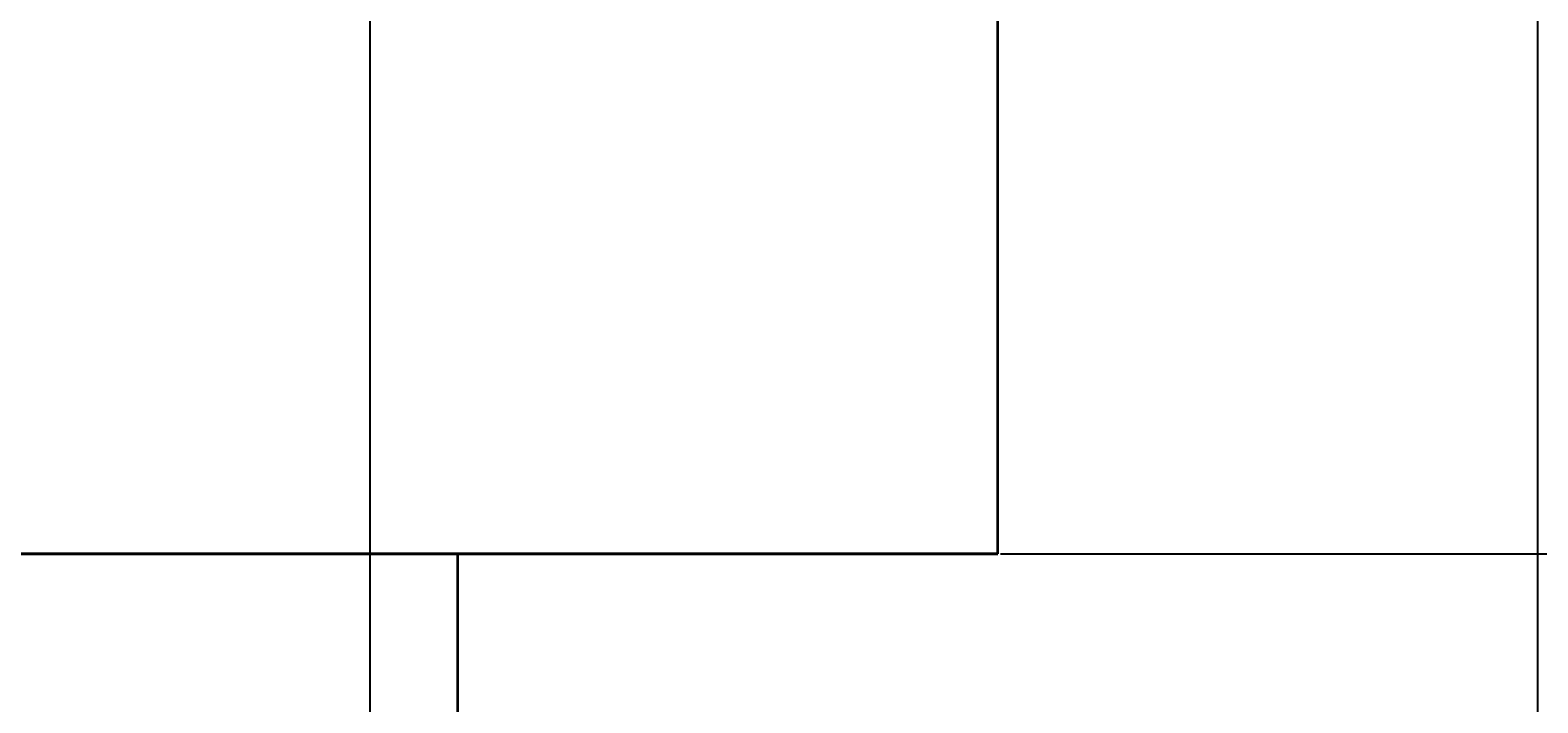
# Model space of a CAD drawing. Units: inches. Extents: x -6 to 289, y -8 to 323.
# Tile 64 of 107: x 238 to 271, y 124 to 139. Entities that reach past the tile are written whole.
import ezdxf

# ---------------------------------------------------------------- set-up
doc = ezdxf.new("R2010")
doc.units = ezdxf.units.IN
doc.header["$MEASUREMENT"] = 0
doc.layers.add('A-ANNO-DIMS', color=2, linetype='Continuous', lineweight=18)
doc.layers.add('A-ELEV', color=7, linetype='Continuous', lineweight=35)
doc.styles.get("Standard").update_dxf_attribs({"font": 'arial.ttf'})
doc.dimstyles.get("Standard").update_dxf_attribs({"dimtxt": 0.18, "dimasz": 0.18, "dimexe": 0.18, "dimexo": 0.0625, "dimgap": 0.09, "dimtad": 0, "dimtih": 1, "dimtoh": 1, "dimdec": 4, "dimzin": 0, "dimdsep": 46, "dimtxsty": 'Standard', "dimcen": 0.09, "dimadec": 0, "dimazin": 0, "dimtfac": 1, "dimtdec": 4, "dimtofl": 0, "dimtmove": 0, "dimatfit": 3, "dimfxl": 1, "dimtolj": 1, "dimtzin": 0, "dimarcsym": 0})

# ---------------------------------------------------------------- blocks, each defined once
blk = doc.blocks.new('*D15')
at = {"layer": 'A-ANNO-DIMS', "color": 0, "lineweight": -2, "transparency": 16777216}
for p, q in [((247.164, 162.411), (247.164, 322.969)), ((247.344, 322.789), (258.944, 322.789)), ((270.984, 322.789), (259.384, 322.789)), ((271.164, 7.351), (271.164, 322.969))]:
    blk.add_line(p, q, dxfattribs=at)
at = {"layer": 'A-ANNO-DIMS', "color": 0, "transparency": 16777216}
for points in [[(247.344, 322.819), (247.344, 322.759), (247.164, 322.789)], [(270.984, 322.819), (270.984, 322.759), (271.164, 322.789)]]:
    blk.add_solid(points, dxfattribs=at)
at = {"layer": 'Defpoints', "color": 0, "transparency": 16777216}
for p in [(271.164, 322.789), (247.164, 162.348), (271.164, 7.289)]:
    blk.add_point(p, dxfattribs=at)
at = {"layer": 'A-ANNO-DIMS', "color": 0, "transparency": 16777216, "insert": (259.164, 322.789), "char_height": 0.18, "attachment_point": 5}
blk.add_mtext('\\A1;24', dxfattribs=at)
blk = doc.blocks.new('*D23')
at = {"layer": 'A-ANNO-DIMS', "color": 0, "lineweight": -2, "transparency": 16777216}
for p, q in [((259.226, 127.289), (288.653, 127.289)), ((288.473, 127.109), (288.473, 67.471)), ((288.473, 7.469), (288.473, 67.107)), ((271.226, 7.289), (288.653, 7.289))]:
    blk.add_line(p, q, dxfattribs=at)
at = {"layer": 'A-ANNO-DIMS', "color": 0, "transparency": 16777216}
for points in [[(288.443, 127.109), (288.503, 127.109), (288.473, 127.289)], [(288.443, 7.469), (288.503, 7.469), (288.473, 7.289)]]:
    blk.add_solid(points, dxfattribs=at)
at = {"layer": 'Defpoints', "color": 0, "transparency": 16777216}
for p in [(259.164, 127.289), (288.473, 127.289), (271.164, 7.289)]:
    blk.add_point(p, dxfattribs=at)
at = {"layer": 'A-ANNO-DIMS', "color": 0, "transparency": 16777216, "insert": (288.473, 67.289), "char_height": 0.18, "attachment_point": 5}
blk.add_mtext('\\A1;120', dxfattribs=at)
blk = doc.blocks.new('*D81')
at = {"layer": 'A-ANNO-DIMS', "color": 0, "lineweight": -2, "transparency": 16777216}
for p, q in [((230.292, 68.842), (230.292, 322.969)), ((230.472, 322.789), (237.298, 322.789)), ((245.035, 322.789), (238.208, 322.789)), ((245.215, 66.286), (245.215, 322.969))]:
    blk.add_line(p, q, dxfattribs=at)
at = {"layer": 'A-ANNO-DIMS', "color": 0, "transparency": 16777216}
for points in [[(230.472, 322.819), (230.472, 322.759), (230.292, 322.789)], [(245.035, 322.819), (245.035, 322.759), (245.215, 322.789)]]:
    blk.add_solid(points, dxfattribs=at)
at = {"layer": 'Defpoints', "color": 0, "transparency": 16777216}
for p in [(245.215, 322.789), (230.292, 68.779), (245.215, 66.224)]:
    blk.add_point(p, dxfattribs=at)
at = {"layer": 'A-ANNO-DIMS', "color": 0, "transparency": 16777216, "insert": (237.753, 322.789), "char_height": 0.18, "attachment_point": 5}
blk.add_mtext('\\A1;14.923', dxfattribs=at)
blk = doc.blocks.new('*D82')
at = {"layer": 'A-ANNO-DIMS', "color": 0, "lineweight": -2, "transparency": 16777216}
for p, q in [((245.215, 66.286), (245.215, 322.969)), ((245.395, 322.789), (258.699, 322.789)), ((272.793, 322.789), (259.489, 322.789)), ((272.973, 66.286), (272.973, 322.969))]:
    blk.add_line(p, q, dxfattribs=at)
at = {"layer": 'A-ANNO-DIMS', "color": 0, "transparency": 16777216}
for points in [[(245.395, 322.819), (245.395, 322.759), (245.215, 322.789)], [(272.793, 322.819), (272.793, 322.759), (272.973, 322.789)]]:
    blk.add_solid(points, dxfattribs=at)
at = {"layer": 'Defpoints', "color": 0, "transparency": 16777216}
for p in [(272.973, 322.789), (245.215, 66.224), (272.973, 66.224)]:
    blk.add_point(p, dxfattribs=at)
at = {"layer": 'A-ANNO-DIMS', "color": 0, "transparency": 16777216, "insert": (259.094, 322.789), "char_height": 0.18, "attachment_point": 5}
blk.add_mtext('\\A1;27.76', dxfattribs=at)
blk = doc.blocks.new('*D101')
at = {"layer": 'A-ANNO-DIMS', "color": 0, "lineweight": -2, "transparency": 16777216}
for p, q in [((259.226, 139.289), (288.653, 139.289)), ((288.473, 139.109), (288.473, 133.469)), ((288.473, 127.469), (288.473, 133.108)), ((259.226, 127.289), (288.653, 127.289))]:
    blk.add_line(p, q, dxfattribs=at)
at = {"layer": 'A-ANNO-DIMS', "color": 0, "transparency": 16777216}
for points in [[(288.443, 139.109), (288.503, 139.109), (288.473, 139.289)], [(288.443, 127.469), (288.503, 127.469), (288.473, 127.289)]]:
    blk.add_solid(points, dxfattribs=at)
at = {"layer": 'Defpoints', "color": 0, "transparency": 16777216}
for p in [(259.164, 139.289), (288.473, 139.289), (259.164, 127.289)]:
    blk.add_point(p, dxfattribs=at)
at = {"layer": 'A-ANNO-DIMS', "color": 0, "transparency": 16777216, "insert": (288.473, 133.289), "char_height": 0.18, "attachment_point": 5}
blk.add_mtext('\\A1;12', dxfattribs=at)

msp = doc.modelspace()

# ---------------------------------------------------------------- linework, layer by layer
at = {"layer": 'A-ELEV'}
for p, q in [((259.1638, 127.2888), (259.1638, 139.2888)), ((259.1638, 127.2888), (115.1638, 127.2888)), ((115.1638, 127.2888), (259.1638, 127.2888)), ((247.1638, 68.4323), (247.1638, 127.2888))]:
    msp.add_line(p, q, dxfattribs=at)

# ---------------------------------------------------------------- dimensions: what is measured, and where the dimension line sits
at = {"layer": 'A-ANNO-DIMS'}
for base, p1, p2, override, picture, middle in [((245.2146, 322.7888), (230.2918, 68.7795), (245.2146, 66.2238), {"dimdec": 3, "dimlfac": 1, "dimrnd": 0, "dimzin": 0, "dimdsep": 46, "dimlunit": 2}, '*D81', (237.7532, 322.7888)), ((272.9733, 322.7888), (245.2146, 66.2238), (272.9733, 66.2238), {"dimdec": 2, "dimlfac": 1, "dimrnd": 0, "dimzin": 0, "dimdsep": 46, "dimlunit": 2}, '*D82', (259.0939, 322.7888)), ((271.1638, 322.7888), (247.1638, 162.3484), (271.1638, 7.2888), {"dimdec": 0, "dimlfac": 1, "dimrnd": 0, "dimzin": 0, "dimdsep": 46, "dimlunit": 2}, '*D15', (259.1638, 322.7888))]:
    dim = msp.add_linear_dim(base=base, p1=p1, p2=p2, dimstyle='Standard', override=override, dxfattribs=at)
    dim.commit()
    dim.dimension.update_dxf_attribs({"geometry": picture, "text_midpoint": middle})
for base, p1, p2, picture, middle in [((288.4733, 139.2888), (259.1638, 127.2888), (259.1638, 139.2888), '*D101', (288.4733, 133.2888)), ((288.4733, 127.2888), (271.1638, 7.2888), (259.1638, 127.2888), '*D23', (288.4733, 67.2888))]:
    dim = msp.add_linear_dim(base=base, p1=p1, p2=p2, angle=90, dimstyle='Standard', override={"dimdec": 0, "dimlfac": 1, "dimrnd": 0, "dimzin": 0, "dimdsep": 46, "dimlunit": 2}, dxfattribs=at)
    dim.commit()
    dim.dimension.update_dxf_attribs({"geometry": picture, "text_midpoint": middle})

doc.saveas('drawing.dxf')
